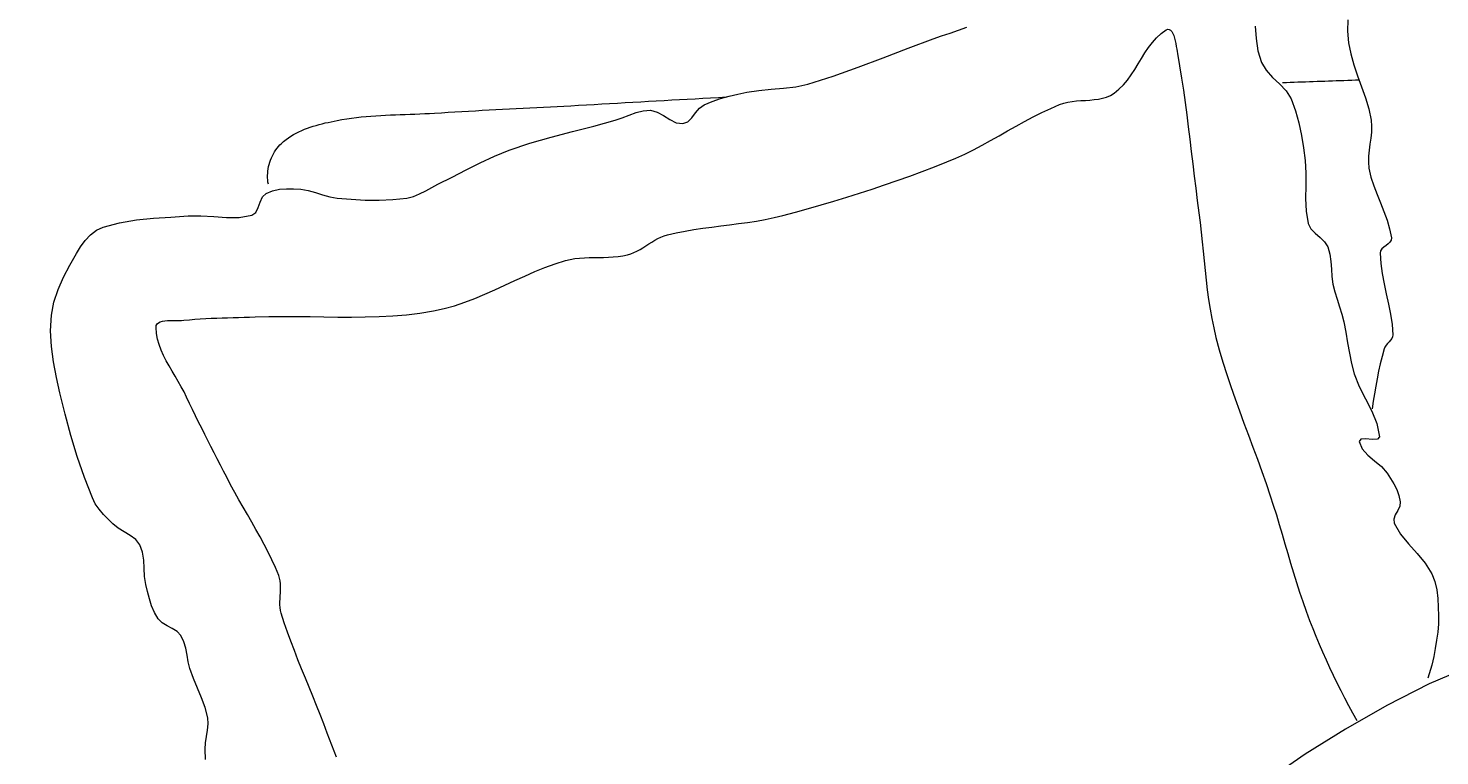
# Model space of a CAD drawing. Units: inches. Extents: x 1441 to 2460, y 1648 to 2683.
# Tile 26 of 35: x 1810 to 1840, y 2268 to 2284. Entities that reach past the tile are written whole.
import ezdxf

# ---------------------------------------------------------------- set-up
doc = ezdxf.new("R2010")
doc.units = ezdxf.units.IN
doc.layers.add('A-ANNO-DIMS', color=2, linetype='Continuous', lineweight=18)
doc.layers.add('A-FURN', color=8, linetype='Continuous', lineweight=15)
doc.styles.get("Standard").update_dxf_attribs({"font": 'arial.ttf'})
doc.dimstyles.get("Standard").update_dxf_attribs({"dimtxt": 0.18, "dimasz": 0.18, "dimexe": 0.18, "dimexo": 0.0625, "dimgap": 0.09, "dimtad": 0, "dimtih": 1, "dimtoh": 1, "dimdec": 4, "dimzin": 0, "dimdsep": 46, "dimtxsty": 'Standard', "dimcen": 0.09, "dimadec": 0, "dimazin": 0, "dimtfac": 1, "dimtdec": 4, "dimtofl": 0, "dimtmove": 0, "dimatfit": 3, "dimfxl": 1, "dimtolj": 1, "dimtzin": 0, "dimarcsym": 0})

# ---------------------------------------------------------------- blocks, each defined once
blk = doc.blocks.new('BED-DOUBLE-PLAN')
for p, q in [((29.214, 88.073), (29.208, 87.829)), ((19.771, 87.466), (20.309, 87.666)), ((20.309, 87.666), (20.489, 87.729)), ((20.489, 87.729), (20.67, 87.789)), ((20.67, 87.789), (20.851, 87.851)), ((20.851, 87.851), (21.031, 87.917)), ((25.019, 87.589), (25.108, 87.69)), ((25.108, 87.69), (25.206, 87.78)), ((25.206, 87.78), (25.316, 87.859)), ((25.316, 87.859), (25.351, 87.873)), ((25.351, 87.873), (25.382, 87.87)), ((25.382, 87.87), (25.41, 87.854)), ((25.41, 87.854), (25.435, 87.824)), ((25.435, 87.824), (25.457, 87.785)), ((25.457, 87.785), (25.476, 87.737)), ((25.476, 87.737), (25.493, 87.683)), ((25.493, 87.683), (25.508, 87.626)), ((27.223, 87.936), (27.246, 87.672)), ((27.246, 87.672), (27.284, 87.412)), ((29.208, 87.829), (29.229, 87.585)), ((19.236, 87.259), (19.771, 87.466)), ((24.785, 87.248), (24.859, 87.366)), ((24.859, 87.366), (24.936, 87.481)), ((24.936, 87.481), (25.019, 87.589)), ((25.508, 87.626), (25.521, 87.566)), ((25.521, 87.566), (25.532, 87.506)), ((25.532, 87.506), (25.542, 87.449)), ((25.542, 87.449), (25.551, 87.396)), ((25.551, 87.396), (25.559, 87.349)), ((25.559, 87.349), (25.604, 87.088)), ((27.284, 87.412), (27.359, 87.162)), ((29.229, 87.585), (29.278, 87.345)), ((29.278, 87.345), (29.347, 87.108)), ((18.16, 86.865), (18.7, 87.056)), ((18.7, 87.056), (19.236, 87.259)), ((24.638, 87.01), (24.712, 87.129)), ((24.712, 87.129), (24.785, 87.248)), ((25.604, 87.088), (25.646, 86.826)), ((27.359, 87.162), (27.462, 86.991)), ((29.347, 87.108), (29.428, 86.873)), ((17.613, 86.694), (18.16, 86.865)), ((24.394, 86.678), (24.481, 86.782)), ((24.481, 86.782), (24.562, 86.894)), ((24.562, 86.894), (24.638, 87.01)), ((25.646, 86.826), (25.684, 86.564)), ((27.462, 86.991), (27.601, 86.84)), ((27.601, 86.84), (27.752, 86.698)), ((27.813, 86.729), (27.896, 86.732)), ((27.896, 86.732), (27.979, 86.735)), ((27.979, 86.735), (28.061, 86.738)), ((28.061, 86.738), (28.144, 86.741)), ((28.144, 86.741), (28.226, 86.744)), ((28.226, 86.744), (28.309, 86.746)), ((28.309, 86.746), (28.391, 86.749)), ((28.391, 86.749), (28.474, 86.752)), ((28.474, 86.752), (28.556, 86.755)), ((28.556, 86.755), (28.639, 86.758)), ((28.639, 86.758), (28.722, 86.761)), ((28.722, 86.761), (28.804, 86.764)), ((28.804, 86.764), (28.887, 86.767)), ((28.887, 86.767), (28.969, 86.77)), ((28.969, 86.77), (29.052, 86.772)), ((29.052, 86.772), (29.134, 86.775)), ((29.134, 86.775), (29.217, 86.778)), ((29.217, 86.778), (29.3, 86.781)), ((29.3, 86.781), (29.382, 86.784)), ((29.382, 86.784), (29.465, 86.787)), ((29.428, 86.873), (29.514, 86.638)), ((15.741, 86.387), (15.927, 86.438)), ((15.927, 86.438), (16.114, 86.481)), ((16.114, 86.481), (16.302, 86.52)), ((16.302, 86.52), (16.564, 86.559)), ((16.564, 86.559), (16.828, 86.583)), ((16.828, 86.583), (17.093, 86.605)), ((17.093, 86.605), (17.356, 86.638)), ((17.356, 86.638), (17.613, 86.694)), ((24.034, 86.417), (24.116, 86.452)), ((24.116, 86.452), (24.194, 86.499)), ((24.194, 86.499), (24.299, 86.583)), ((24.299, 86.583), (24.394, 86.678)), ((25.684, 86.564), (25.721, 86.301)), ((27.752, 86.698), (27.893, 86.548)), ((27.893, 86.548), (28, 86.378)), ((29.514, 86.638), (29.596, 86.402)), ((10.474, 86.124), (10.62, 86.132)), ((10.62, 86.132), (10.767, 86.14)), ((10.767, 86.14), (10.913, 86.147)), ((10.913, 86.147), (11.059, 86.155)), ((11.059, 86.155), (11.206, 86.163)), ((11.206, 86.163), (11.352, 86.17)), ((11.352, 86.17), (11.499, 86.178)), ((11.499, 86.178), (11.645, 86.185)), ((11.645, 86.185), (11.792, 86.193)), ((11.792, 86.193), (11.938, 86.201)), ((11.938, 86.201), (12.085, 86.209)), ((12.085, 86.209), (12.231, 86.216)), ((12.231, 86.216), (12.377, 86.224)), ((12.377, 86.224), (12.524, 86.232)), ((12.524, 86.232), (12.691, 86.242)), ((12.691, 86.242), (12.858, 86.251)), ((12.858, 86.251), (13.024, 86.26)), ((13.024, 86.26), (13.191, 86.27)), ((13.191, 86.27), (13.358, 86.279)), ((13.358, 86.279), (13.525, 86.288)), ((13.525, 86.288), (13.692, 86.298)), ((13.692, 86.298), (13.859, 86.307)), ((13.859, 86.307), (14.025, 86.316)), ((14.025, 86.316), (14.192, 86.326)), ((14.077, 86.121), (14.232, 86.132)), ((14.192, 86.326), (14.359, 86.335)), ((14.232, 86.132), (14.378, 86.095)), ((14.359, 86.335), (14.526, 86.344)), ((14.526, 86.344), (14.693, 86.354)), ((14.693, 86.354), (14.859, 86.363)), ((14.859, 86.363), (15.026, 86.373)), ((15.026, 86.373), (15.193, 86.382)), ((15.193, 86.382), (15.36, 86.392)), ((15.205, 86.075), (15.287, 86.175)), ((15.287, 86.175), (15.385, 86.249)), ((15.36, 86.392), (15.527, 86.401)), ((15.385, 86.249), (15.56, 86.325)), ((15.527, 86.401), (15.694, 86.411)), ((15.56, 86.325), (15.741, 86.387)), ((15.694, 86.411), (15.86, 86.42)), ((22.646, 86.085), (22.835, 86.174)), ((22.835, 86.174), (23.026, 86.257)), ((23.026, 86.257), (23.113, 86.287)), ((23.113, 86.287), (23.203, 86.309)), ((23.203, 86.309), (23.295, 86.324)), ((23.295, 86.324), (23.389, 86.334)), ((23.389, 86.334), (23.483, 86.34)), ((23.483, 86.34), (23.578, 86.346)), ((23.578, 86.346), (23.673, 86.352)), ((23.673, 86.352), (23.767, 86.361)), ((23.767, 86.361), (23.858, 86.373)), ((23.858, 86.373), (23.948, 86.391)), ((23.948, 86.391), (24.034, 86.417)), ((25.721, 86.301), (25.756, 86.038)), ((28, 86.378), (28.096, 86.124)), ((29.596, 86.402), (29.666, 86.164)), ((29.666, 86.164), (29.717, 85.922)), ((7.053, 85.809), (7.117, 85.827)), ((7.117, 85.827), (7.181, 85.844)), ((7.181, 85.844), (7.246, 85.86)), ((7.246, 85.86), (7.31, 85.874)), ((7.31, 85.874), (7.374, 85.888)), ((7.374, 85.888), (7.438, 85.902)), ((7.438, 85.902), (7.502, 85.915)), ((7.502, 85.915), (7.605, 85.934)), ((7.605, 85.934), (7.709, 85.951)), ((7.709, 85.951), (7.812, 85.966)), ((7.812, 85.966), (7.916, 85.979)), ((7.916, 85.979), (8.021, 85.99)), ((8.021, 85.99), (8.125, 86)), ((8.125, 86), (8.23, 86.008)), ((8.23, 86.008), (8.334, 86.016)), ((8.334, 86.016), (8.439, 86.022)), ((8.439, 86.022), (8.544, 86.028)), ((8.544, 86.028), (8.649, 86.032)), ((8.649, 86.032), (8.755, 86.037)), ((8.755, 86.037), (8.86, 86.04)), ((8.86, 86.04), (8.965, 86.044)), ((8.965, 86.044), (9.07, 86.048)), ((9.07, 86.048), (9.175, 86.052)), ((9.175, 86.052), (9.281, 86.056)), ((9.281, 86.056), (9.386, 86.061)), ((9.386, 86.061), (9.491, 86.066)), ((9.491, 86.066), (9.595, 86.072)), ((9.595, 86.072), (9.742, 86.081)), ((9.742, 86.081), (9.888, 86.09)), ((9.888, 86.09), (10.035, 86.099)), ((10.035, 86.099), (10.181, 86.107)), ((10.181, 86.107), (10.327, 86.116)), ((10.327, 86.116), (10.474, 86.124)), ((13.016, 85.794), (13.473, 85.918)), ((13.473, 85.918), (13.624, 85.969)), ((13.624, 85.969), (13.774, 86.028)), ((13.774, 86.028), (13.925, 86.082)), ((13.925, 86.082), (14.077, 86.121)), ((14.378, 86.095), (14.515, 86.019)), ((14.515, 86.019), (14.65, 85.933)), ((14.65, 85.933), (14.788, 85.865)), ((14.788, 85.865), (14.932, 85.847)), ((14.932, 85.847), (15.039, 85.888)), ((15.039, 85.888), (15.126, 85.971)), ((15.126, 85.971), (15.205, 86.075)), ((22.091, 85.792), (22.274, 85.893)), ((22.274, 85.893), (22.459, 85.991)), ((22.459, 85.991), (22.646, 86.085)), ((25.756, 86.038), (25.789, 85.775)), ((28.096, 86.124), (28.167, 85.862)), ((28.167, 85.862), (28.22, 85.594)), ((29.717, 85.922), (29.728, 85.794)), ((6.405, 85.506), (6.457, 85.544)), ((6.457, 85.544), (6.511, 85.579)), ((6.511, 85.579), (6.567, 85.612)), ((6.567, 85.612), (6.624, 85.643)), ((6.624, 85.643), (6.682, 85.672)), ((6.682, 85.672), (6.742, 85.699)), ((6.742, 85.699), (6.802, 85.724)), ((6.802, 85.724), (6.864, 85.748)), ((6.864, 85.748), (6.926, 85.77)), ((6.926, 85.77), (6.989, 85.79)), ((6.989, 85.79), (7.053, 85.809)), ((11.645, 85.425), (12.1, 85.556)), ((12.1, 85.556), (12.558, 85.676)), ((12.558, 85.676), (13.016, 85.794)), ((21.542, 85.485), (21.725, 85.587)), ((21.725, 85.587), (21.908, 85.69)), ((21.908, 85.69), (22.091, 85.792)), ((25.789, 85.775), (25.821, 85.511)), ((28.22, 85.594), (28.261, 85.323)), ((29.71, 85.536), (29.692, 85.406)), ((29.724, 85.665), (29.71, 85.536)), ((29.728, 85.794), (29.724, 85.665)), ((6.134, 85.199), (6.158, 85.24)), ((6.158, 85.24), (6.184, 85.281)), ((6.184, 85.281), (6.212, 85.319)), ((6.212, 85.319), (6.241, 85.356)), ((6.241, 85.356), (6.273, 85.391)), ((6.273, 85.391), (6.306, 85.423)), ((6.306, 85.423), (6.354, 85.466)), ((6.354, 85.466), (6.405, 85.506)), ((10.883, 85.149), (11.197, 85.276)), ((11.197, 85.276), (11.645, 85.425)), ((20.986, 85.194), (21.173, 85.287)), ((21.173, 85.287), (21.358, 85.385)), ((21.358, 85.385), (21.542, 85.485)), ((25.821, 85.511), (25.853, 85.248)), ((25.853, 85.248), (25.884, 84.984)), ((28.261, 85.323), (28.298, 85.053)), ((29.674, 85.276), (29.661, 85.147)), ((29.692, 85.406), (29.674, 85.276)), ((6.023, 84.877), (6.032, 84.924)), ((6.032, 84.924), (6.044, 84.972)), ((6.044, 84.972), (6.057, 85.019)), ((6.057, 85.019), (6.073, 85.065)), ((6.073, 85.065), (6.092, 85.111)), ((6.092, 85.111), (6.112, 85.155)), ((6.112, 85.155), (6.134, 85.199)), ((10.274, 84.851), (10.576, 85.005)), ((10.576, 85.005), (10.883, 85.149)), ((20.072, 84.818), (20.338, 84.92)), ((20.338, 84.92), (20.604, 85.025)), ((20.604, 85.025), (20.796, 85.106)), ((20.796, 85.106), (20.986, 85.194)), ((25.884, 84.984), (25.915, 84.72)), ((28.298, 85.053), (28.318, 84.783)), ((29.661, 85.147), (29.658, 85.018)), ((29.658, 85.018), (29.671, 84.89)), ((6.009, 84.732), (6.011, 84.78)), ((6.009, 84.685), (6.009, 84.732)), ((6.012, 84.638), (6.009, 84.685)), ((6.011, 84.78), (6.015, 84.828)), ((6.017, 84.591), (6.012, 84.638)), ((6.015, 84.828), (6.023, 84.877)), ((9.668, 84.546), (9.972, 84.695)), ((9.972, 84.695), (10.274, 84.851)), ((19.265, 84.529), (19.535, 84.623)), ((19.535, 84.623), (19.804, 84.719)), ((19.804, 84.719), (20.072, 84.818)), ((25.915, 84.72), (25.948, 84.457)), ((28.318, 84.783), (28.316, 84.51)), ((29.671, 84.89), (29.714, 84.699)), ((29.714, 84.699), (29.774, 84.511)), ((5.898, 84.271), (5.976, 84.349)), ((5.976, 84.349), (6.115, 84.405)), ((6.025, 84.546), (6.017, 84.591)), ((6.115, 84.405), (6.262, 84.436)), ((6.262, 84.436), (6.415, 84.448)), ((6.415, 84.448), (6.569, 84.447)), ((6.569, 84.447), (6.721, 84.438)), ((6.721, 84.438), (6.88, 84.413)), ((6.88, 84.413), (7.036, 84.368)), ((7.036, 84.368), (7.192, 84.317)), ((7.192, 84.317), (7.348, 84.271)), ((9.141, 84.279), (9.276, 84.335)), ((9.276, 84.335), (9.407, 84.405)), ((9.407, 84.405), (9.537, 84.478)), ((9.537, 84.478), (9.668, 84.546)), ((18.451, 84.264), (18.723, 84.35)), ((18.723, 84.35), (18.995, 84.438)), ((18.995, 84.438), (19.265, 84.529)), ((25.948, 84.457), (25.981, 84.194)), ((28.316, 84.51), (28.311, 84.238)), ((29.774, 84.511), (29.844, 84.326)), ((29.844, 84.326), (29.919, 84.142)), ((5.753, 83.94), (5.807, 84.042)), ((5.807, 84.042), (5.848, 84.161)), ((5.848, 84.161), (5.898, 84.271)), ((7.348, 84.271), (7.507, 84.244)), ((7.507, 84.244), (7.806, 84.221)), ((7.806, 84.221), (8.105, 84.206)), ((8.105, 84.206), (8.405, 84.203)), ((8.405, 84.203), (8.703, 84.214)), ((8.703, 84.214), (9, 84.245)), ((9, 84.245), (9.141, 84.279)), ((17.353, 83.946), (17.629, 84.022)), ((17.629, 84.022), (17.903, 84.1)), ((17.903, 84.1), (18.177, 84.181)), ((18.177, 84.181), (18.451, 84.264)), ((25.981, 84.194), (26.015, 83.931)), ((28.311, 84.238), (28.322, 83.968)), ((29.919, 84.142), (29.993, 83.958)), ((2.475, 83.624), (2.83, 83.719)), ((2.83, 83.719), (3.193, 83.779)), ((3.193, 83.779), (3.561, 83.814)), ((3.561, 83.814), (3.931, 83.839)), ((3.931, 83.839), (4.3, 83.864)), ((4.3, 83.864), (4.575, 83.867)), ((4.575, 83.867), (4.852, 83.849)), ((4.852, 83.849), (5.128, 83.83)), ((5.128, 83.83), (5.401, 83.833)), ((5.401, 83.833), (5.668, 83.879)), ((5.668, 83.879), (5.753, 83.94)), ((15.935, 83.675), (16.128, 83.699)), ((16.128, 83.699), (16.319, 83.726)), ((16.319, 83.726), (16.51, 83.755)), ((16.51, 83.755), (16.701, 83.789)), ((16.701, 83.789), (16.89, 83.828)), ((16.89, 83.828), (17.078, 83.873)), ((17.078, 83.873), (17.353, 83.946)), ((26.015, 83.931), (26.042, 83.725)), ((26.042, 83.725), (26.065, 83.518)), ((28.322, 83.968), (28.367, 83.704)), ((28.367, 83.704), (28.424, 83.589)), ((29.993, 83.958), (30.06, 83.772)), ((30.06, 83.772), (30.115, 83.584)), ((2.089, 83.333), (2.203, 83.455)), ((2.203, 83.455), (2.331, 83.555)), ((2.331, 83.555), (2.475, 83.624)), ((14.394, 83.376), (14.461, 83.408)), ((14.461, 83.408), (14.529, 83.436)), ((14.529, 83.436), (14.6, 83.457)), ((14.6, 83.457), (14.788, 83.501)), ((14.788, 83.501), (14.977, 83.539)), ((14.977, 83.539), (15.168, 83.572)), ((15.168, 83.572), (15.359, 83.6)), ((15.359, 83.6), (15.551, 83.626)), ((15.551, 83.626), (15.743, 83.651)), ((15.743, 83.651), (15.935, 83.675)), ((26.065, 83.518), (26.087, 83.311)), ((28.424, 83.589), (28.516, 83.493)), ((28.516, 83.493), (28.62, 83.403)), ((28.62, 83.403), (28.718, 83.309)), ((30.115, 83.584), (30.152, 83.392)), ((1.902, 83.059), (1.99, 83.199)), ((1.99, 83.199), (2.089, 83.333)), ((13.878, 83.076), (13.945, 83.108)), ((13.945, 83.108), (14.01, 83.144)), ((14.01, 83.144), (14.074, 83.182)), ((14.074, 83.182), (14.138, 83.222)), ((14.138, 83.222), (14.201, 83.262)), ((14.201, 83.262), (14.265, 83.302)), ((14.265, 83.302), (14.329, 83.341)), ((14.329, 83.341), (14.394, 83.376)), ((26.087, 83.311), (26.108, 83.104)), ((26.108, 83.104), (26.129, 82.897)), ((28.718, 83.309), (28.788, 83.198)), ((28.788, 83.198), (28.833, 83.045)), ((29.921, 83.113), (29.911, 83.066)), ((29.95, 83.155), (29.921, 83.113)), ((29.991, 83.193), (29.95, 83.155)), ((30.037, 83.229), (29.991, 83.193)), ((30.083, 83.265), (30.037, 83.229)), ((30.121, 83.303), (30.083, 83.265)), ((30.146, 83.345), (30.121, 83.303)), ((30.152, 83.392), (30.146, 83.345)), ((1.626, 82.55), (1.759, 82.808)), ((1.759, 82.808), (1.902, 83.059)), ((11.967, 82.755), (12.187, 82.836)), ((12.187, 82.836), (12.409, 82.906)), ((12.409, 82.906), (12.509, 82.931)), ((12.509, 82.931), (12.61, 82.948)), ((12.61, 82.948), (12.711, 82.96)), ((12.711, 82.96), (12.814, 82.967)), ((12.814, 82.967), (12.917, 82.971)), ((12.917, 82.971), (13.021, 82.972)), ((13.021, 82.972), (13.125, 82.973)), ((13.125, 82.973), (13.229, 82.974)), ((13.229, 82.974), (13.332, 82.976)), ((13.332, 82.976), (13.435, 82.982)), ((13.435, 82.982), (13.538, 82.991)), ((13.538, 82.991), (13.639, 83.006)), ((13.639, 83.006), (13.739, 83.027)), ((13.739, 83.027), (13.81, 83.049)), ((13.81, 83.049), (13.878, 83.076)), ((26.129, 82.897), (26.151, 82.689)), ((28.833, 83.045), (28.854, 82.886)), ((28.854, 82.886), (28.863, 82.724)), ((29.911, 83.066), (29.924, 82.845)), ((29.924, 82.845), (29.954, 82.626)), ((1.51, 82.285), (1.626, 82.55)), ((11.321, 82.476), (11.535, 82.573)), ((11.535, 82.573), (11.75, 82.667)), ((11.75, 82.667), (11.967, 82.755)), ((26.151, 82.689), (26.173, 82.483)), ((28.863, 82.724), (28.873, 82.561)), ((28.873, 82.561), (28.896, 82.401)), ((29.954, 82.626), (29.995, 82.407)), ((1.42, 82.012), (1.51, 82.285)), ((10.464, 82.093), (10.679, 82.183)), ((10.679, 82.183), (10.894, 82.279)), ((10.894, 82.279), (11.108, 82.377)), ((11.108, 82.377), (11.321, 82.476)), ((26.173, 82.483), (26.198, 82.276)), ((26.198, 82.276), (26.226, 82.07)), ((28.896, 82.401), (28.937, 82.237)), ((28.937, 82.237), (28.985, 82.075)), ((29.995, 82.407), (30.042, 82.189)), ((30.042, 82.189), (30.09, 81.971)), ((1.366, 81.731), (1.42, 82.012)), ((9.802, 81.873), (10.026, 81.936)), ((10.026, 81.936), (10.246, 82.01)), ((10.246, 82.01), (10.464, 82.093)), ((26.226, 82.07), (26.258, 81.865)), ((28.985, 82.075), (29.036, 81.914)), ((29.036, 81.914), (29.086, 81.753)), ((30.09, 81.971), (30.133, 81.753)), ((1.348, 81.397), (1.366, 81.731)), ((3.665, 81.569), (3.704, 81.588)), ((3.704, 81.588), (3.751, 81.602)), ((3.751, 81.602), (3.804, 81.61)), ((3.804, 81.61), (3.862, 81.615)), ((3.862, 81.615), (3.922, 81.618)), ((3.922, 81.618), (3.984, 81.618)), ((3.984, 81.618), (4.046, 81.618)), ((4.046, 81.618), (4.106, 81.618)), ((4.106, 81.618), (4.162, 81.619)), ((4.162, 81.619), (4.212, 81.623)), ((4.212, 81.623), (4.329, 81.634)), ((4.329, 81.634), (4.446, 81.644)), ((4.446, 81.644), (4.564, 81.652)), ((4.564, 81.652), (4.681, 81.659)), ((4.681, 81.659), (4.798, 81.665)), ((4.798, 81.665), (4.916, 81.67)), ((4.916, 81.67), (5.033, 81.674)), ((5.033, 81.674), (5.151, 81.678)), ((5.151, 81.678), (5.269, 81.681)), ((5.269, 81.681), (5.386, 81.684)), ((5.386, 81.684), (5.504, 81.688)), ((5.504, 81.688), (5.621, 81.691)), ((5.621, 81.691), (5.739, 81.695)), ((5.739, 81.695), (6.034, 81.703)), ((6.034, 81.703), (6.33, 81.706)), ((6.33, 81.706), (6.626, 81.704)), ((6.626, 81.704), (6.923, 81.701)), ((6.923, 81.701), (7.219, 81.696)), ((7.219, 81.696), (7.516, 81.693)), ((7.516, 81.693), (7.812, 81.692)), ((7.812, 81.692), (8.108, 81.695)), ((8.108, 81.695), (8.403, 81.703)), ((8.403, 81.703), (8.697, 81.719)), ((8.697, 81.719), (8.991, 81.743)), ((8.991, 81.743), (9.283, 81.778)), ((9.283, 81.778), (9.574, 81.824)), ((9.574, 81.824), (9.802, 81.873)), ((26.258, 81.865), (26.294, 81.661)), ((26.294, 81.661), (26.335, 81.458)), ((29.086, 81.753), (29.129, 81.589)), ((29.129, 81.589), (29.175, 81.367)), ((30.133, 81.753), (30.166, 81.534)), ((1.367, 81.062), (1.348, 81.397)), ((3.612, 81.466), (3.617, 81.509)), ((3.623, 81.342), (3.612, 81.466)), ((3.617, 81.509), (3.635, 81.543)), ((3.646, 81.22), (3.623, 81.342)), ((3.635, 81.543), (3.665, 81.569)), ((26.335, 81.458), (26.383, 81.256)), ((29.175, 81.367), (29.213, 81.142)), ((30.166, 81.534), (30.185, 81.313)), ((30.185, 81.313), (30.179, 81.27)), ((1.413, 80.727), (1.367, 81.062)), ((3.68, 81.101), (3.646, 81.22)), ((3.723, 80.984), (3.68, 81.101)), ((3.774, 80.869), (3.723, 80.984)), ((26.383, 81.256), (26.454, 80.989)), ((26.454, 80.989), (26.531, 80.724)), ((29.213, 81.142), (29.25, 80.917)), ((29.996, 81.006), (29.954, 80.848)), ((30.014, 81.048), (29.996, 81.006)), ((30.04, 81.086), (30.014, 81.048)), ((30.071, 81.123), (30.04, 81.086)), ((30.104, 81.158), (30.071, 81.123)), ((30.136, 81.194), (30.104, 81.158)), ((30.162, 81.231), (30.136, 81.194)), ((30.179, 81.27), (30.162, 81.231)), ((1.477, 80.394), (1.413, 80.727)), ((3.831, 80.755), (3.774, 80.869)), ((3.892, 80.643), (3.831, 80.755)), ((26.531, 80.724), (26.614, 80.46)), ((29.25, 80.917), (29.294, 80.695)), ((29.294, 80.695), (29.352, 80.475)), ((29.915, 80.689), (29.879, 80.529)), ((29.954, 80.848), (29.915, 80.689)), ((1.549, 80.065), (1.477, 80.394)), ((3.957, 80.531), (3.892, 80.643)), ((4.023, 80.419), (3.957, 80.531)), ((4.088, 80.308), (4.023, 80.419)), ((26.614, 80.46), (26.702, 80.198)), ((29.352, 80.475), (29.461, 80.202)), ((29.846, 80.368), (29.815, 80.207)), ((29.879, 80.529), (29.846, 80.368)), ((1.659, 79.605), (1.549, 80.065)), ((4.153, 80.196), (4.088, 80.308)), ((4.214, 80.084), (4.153, 80.196)), ((4.27, 79.971), (4.214, 80.084)), ((26.702, 80.198), (26.793, 79.936)), ((29.461, 80.202), (29.597, 79.937)), ((29.815, 80.207), (29.788, 80.045)), ((4.334, 79.837), (4.27, 79.971)), ((4.398, 79.704), (4.334, 79.837)), ((26.793, 79.936), (26.887, 79.676)), ((29.597, 79.937), (29.734, 79.673)), ((29.764, 79.883), (29.743, 79.721)), ((29.788, 80.045), (29.764, 79.883)), ((1.783, 79.148), (1.659, 79.605)), ((4.462, 79.571), (4.398, 79.704)), ((4.527, 79.438), (4.462, 79.571)), ((26.887, 79.676), (26.983, 79.416)), ((29.734, 79.673), (29.843, 79.403)), ((4.593, 79.305), (4.527, 79.438)), ((4.659, 79.173), (4.593, 79.305)), ((4.725, 79.041), (4.659, 79.173)), ((26.983, 79.416), (27.08, 79.157)), ((27.08, 79.157), (27.177, 78.897)), ((29.843, 79.403), (29.9, 79.12)), ((1.921, 78.696), (1.783, 79.148)), ((4.792, 78.909), (4.725, 79.041)), ((4.859, 78.777), (4.792, 78.909)), ((27.177, 78.897), (27.274, 78.638)), ((29.494, 79.073), (29.458, 79.021)), ((29.458, 79.021), (29.528, 78.86)), ((29.604, 79.076), (29.494, 79.073)), ((29.528, 78.86), (29.648, 78.726)), ((29.741, 79.063), (29.604, 79.076)), ((29.856, 79.066), (29.741, 79.063)), ((29.9, 79.12), (29.856, 79.066)), ((2.075, 78.248), (1.921, 78.696)), ((4.927, 78.645), (4.859, 78.777)), ((4.994, 78.513), (4.927, 78.645)), ((27.274, 78.638), (27.368, 78.377)), ((29.648, 78.726), (29.793, 78.603)), ((29.793, 78.603), (29.939, 78.48)), ((2.244, 77.807), (2.075, 78.248)), ((5.062, 78.382), (4.994, 78.513)), ((5.13, 78.25), (5.062, 78.382)), ((5.215, 78.088), (5.13, 78.25)), ((27.368, 78.377), (27.461, 78.116)), ((29.939, 78.48), (30.061, 78.342)), ((30.061, 78.342), (30.137, 78.228)), ((5.304, 77.927), (5.215, 78.088)), ((27.461, 78.116), (27.55, 77.854)), ((30.137, 78.228), (30.206, 78.109)), ((30.206, 78.109), (30.267, 77.986)), ((30.267, 77.986), (30.314, 77.859)), ((2.307, 77.68), (2.244, 77.807)), ((2.388, 77.564), (2.307, 77.68)), ((5.394, 77.767), (5.304, 77.927)), ((5.485, 77.608), (5.394, 77.767)), ((27.55, 77.854), (27.616, 77.649)), ((27.616, 77.649), (27.681, 77.442)), ((30.314, 77.859), (30.343, 77.727)), ((30.343, 77.727), (30.332, 77.631)), ((2.481, 77.454), (2.388, 77.564)), ((2.582, 77.35), (2.481, 77.454)), ((2.684, 77.249), (2.582, 77.35)), ((5.577, 77.449), (5.485, 77.608)), ((5.669, 77.289), (5.577, 77.449)), ((27.681, 77.442), (27.743, 77.235)), ((30.237, 77.443), (30.203, 77.351)), ((30.203, 77.351), (30.212, 77.262)), ((30.288, 77.537), (30.237, 77.443)), ((30.332, 77.631), (30.288, 77.537)), ((2.8, 77.157), (2.684, 77.249)), ((2.929, 77.079), (2.8, 77.157)), ((3.059, 77.002), (2.929, 77.079)), ((5.759, 77.13), (5.669, 77.289)), ((5.849, 76.969), (5.759, 77.13)), ((27.743, 77.235), (27.805, 77.028)), ((27.805, 77.028), (27.866, 76.82)), ((30.212, 77.262), (30.347, 77.03)), ((30.347, 77.03), (30.518, 76.819)), ((3.175, 76.914), (3.059, 77.002)), ((3.263, 76.801), (3.175, 76.914)), ((3.323, 76.643), (3.263, 76.801)), ((5.936, 76.808), (5.849, 76.969)), ((6.02, 76.645), (5.936, 76.808)), ((27.866, 76.82), (27.927, 76.612)), ((30.518, 76.819), (30.704, 76.617)), ((3.348, 76.473), (3.323, 76.643)), ((3.356, 76.298), (3.348, 76.473)), ((6.1, 76.48), (6.02, 76.645)), ((6.176, 76.314), (6.1, 76.48)), ((27.927, 76.612), (27.988, 76.405)), ((30.704, 76.617), (30.879, 76.408)), ((3.364, 76.122), (3.356, 76.298)), ((3.391, 75.951), (3.364, 76.122)), ((6.247, 76.145), (6.176, 76.314)), ((6.267, 76.086), (6.247, 76.145)), ((27.988, 76.405), (28.051, 76.197)), ((28.051, 76.197), (28.114, 75.991)), ((30.879, 76.408), (31.02, 76.18)), ((31.02, 76.18), (31.086, 76.009)), ((3.428, 75.797), (3.391, 75.951)), ((6.28, 76.025), (6.267, 76.086)), ((6.286, 75.963), (6.28, 76.025)), ((6.285, 75.772), (6.288, 75.836)), ((6.289, 75.9), (6.286, 75.963)), ((6.288, 75.836), (6.289, 75.9)), ((28.114, 75.991), (28.18, 75.785)), ((31.086, 76.009), (31.127, 75.831)), ((31.127, 75.831), (31.15, 75.647)), ((3.469, 75.643), (3.428, 75.797)), ((3.518, 75.492), (3.469, 75.643)), ((6.275, 75.579), (6.277, 75.643)), ((6.275, 75.515), (6.275, 75.579)), ((6.279, 75.452), (6.275, 75.515)), ((6.277, 75.643), (6.281, 75.708)), ((6.281, 75.708), (6.285, 75.772)), ((28.18, 75.785), (28.249, 75.58)), ((28.249, 75.58), (28.321, 75.376)), ((31.15, 75.647), (31.161, 75.461)), ((3.579, 75.347), (3.518, 75.492)), ((3.657, 75.211), (3.579, 75.347)), ((3.742, 75.126), (3.657, 75.211)), ((6.288, 75.39), (6.279, 75.452)), ((6.303, 75.329), (6.288, 75.39)), ((6.367, 75.127), (6.303, 75.329)), ((28.321, 75.376), (28.397, 75.174)), ((31.161, 75.461), (31.167, 75.277)), ((31.167, 75.277), (31.164, 75.101)), ((3.848, 75.061), (3.742, 75.126)), ((3.96, 75.003), (3.848, 75.061)), ((4.064, 74.937), (3.96, 75.003)), ((4.146, 74.85), (4.064, 74.937)), ((6.436, 74.927), (6.367, 75.127)), ((6.508, 74.728), (6.436, 74.927)), ((28.397, 75.174), (28.463, 75.004)), ((28.463, 75.004), (28.532, 74.835)), ((31.148, 74.926), (31.124, 74.751)), ((31.164, 75.101), (31.148, 74.926)), ((4.21, 74.72), (4.146, 74.85)), ((4.25, 74.579), (4.21, 74.72)), ((6.584, 74.53), (6.508, 74.728)), ((28.532, 74.835), (28.602, 74.666)), ((28.602, 74.666), (28.675, 74.499)), ((31.124, 74.751), (31.094, 74.577)), ((4.278, 74.433), (4.25, 74.579)), ((4.304, 74.287), (4.278, 74.433)), ((6.661, 74.333), (6.584, 74.53)), ((6.74, 74.136), (6.661, 74.333)), ((28.675, 74.499), (28.749, 74.332)), ((28.749, 74.332), (28.825, 74.166)), ((31.045, 74.308), (31.023, 74.214)), ((31.064, 74.403), (31.045, 74.308)), ((31.094, 74.577), (31.064, 74.403)), ((4.341, 74.144), (4.304, 74.287)), ((4.419, 73.932), (4.341, 74.144)), ((6.821, 73.94), (6.74, 74.136)), ((28.825, 74.166), (28.903, 74.001)), ((28.903, 74.001), (28.983, 73.837)), ((30.966, 74.029), (30.933, 73.938)), ((31.901, 74.215), (30.964, 73.813)), ((30.996, 74.121), (30.966, 74.029)), ((31.023, 74.214), (30.996, 74.121)), ((4.506, 73.724), (4.419, 73.932)), ((4.592, 73.515), (4.506, 73.724)), ((6.901, 73.744), (6.821, 73.94)), ((6.982, 73.548), (6.901, 73.744)), ((28.983, 73.837), (29.064, 73.674)), ((30.964, 73.813), (30.052, 73.35)), ((4.667, 73.304), (4.592, 73.515)), ((7.062, 73.352), (6.982, 73.548)), ((29.064, 73.674), (29.148, 73.511)), ((29.148, 73.511), (29.233, 73.35)), ((4.722, 73.087), (4.667, 73.304)), ((4.732, 72.953), (4.722, 73.087)), ((7.14, 73.155), (7.062, 73.352)), ((7.216, 72.957), (7.14, 73.155)), ((30.052, 73.35), (29.164, 72.842)), ((29.233, 73.35), (29.32, 73.189)), ((29.32, 73.189), (29.409, 73.03)), ((4.697, 72.682), (4.72, 72.818)), ((4.72, 72.818), (4.732, 72.953)), ((7.289, 72.758), (7.216, 72.957)), ((29.164, 72.842), (28.298, 72.301)), ((4.668, 72.41), (4.675, 72.546)), ((4.675, 72.546), (4.697, 72.682)), ((7.337, 72.628), (7.289, 72.758)), ((7.386, 72.498), (7.337, 72.628)), ((7.436, 72.369), (7.386, 72.498)), ((4.673, 72.189), (4.668, 72.41)), ((7.486, 72.239), (7.436, 72.369)), ((28.298, 72.301), (26.791, 71.264))]:
    blk.add_line(p, q)
blk = doc.blocks.new('*D67')
at = {"layer": 'A-ANNO-DIMS', "color": 0, "lineweight": -2, "transparency": 16777216}
for p, q in [((1889.448, 2298.695), (1916.216, 2298.695)), ((1916.036, 2298.515), (1916.036, 2055.938)), ((1916.036, 1812.997), (1916.036, 2055.574)), ((1758.224, 1812.817), (1916.216, 1812.817))]:
    blk.add_line(p, q, dxfattribs=at)
at = {"layer": 'A-ANNO-DIMS', "color": 0, "transparency": 16777216}
for points in [[(1916.006, 2298.515), (1916.066, 2298.515), (1916.036, 2298.695)], [(1916.006, 1812.997), (1916.066, 1812.997), (1916.036, 1812.817)]]:
    blk.add_solid(points, dxfattribs=at)
at = {"layer": 'Defpoints', "color": 0, "transparency": 16777216}
for p in [(1889.386, 2298.695), (1916.036, 2298.695), (1758.161, 1812.817)]:
    blk.add_point(p, dxfattribs=at)
at = {"layer": 'A-ANNO-DIMS', "color": 0, "transparency": 16777216, "insert": (1916.036, 2055.756), "char_height": 0.18, "attachment_point": 5}
blk.add_mtext('\\A1;485.9', dxfattribs=at)

msp = doc.modelspace()

# ---------------------------------------------------------------- block references
at = {"layer": 'A-FURN'}
msp.add_blockref('BED-DOUBLE-PLAN', (1809.2, 2196.18), dxfattribs=at)

# ---------------------------------------------------------------- dimensions: what is measured, and where the dimension line sits
at = {"layer": 'A-ANNO-DIMS'}
dim = msp.add_linear_dim(base=(1916.0359, 2298.6952), p1=(1758.1615, 1812.8171), p2=(1889.3859, 2298.6952), angle=90, dimstyle='Standard', override={"dimdec": 1, "dimlfac": 1, "dimrnd": 0, "dimzin": 0, "dimdsep": 46, "dimlunit": 2}, dxfattribs=at)
dim.commit()
dim.dimension.update_dxf_attribs({"geometry": '*D67', "text_midpoint": (1916.0359, 2055.7561)})

doc.saveas('drawing.dxf')
